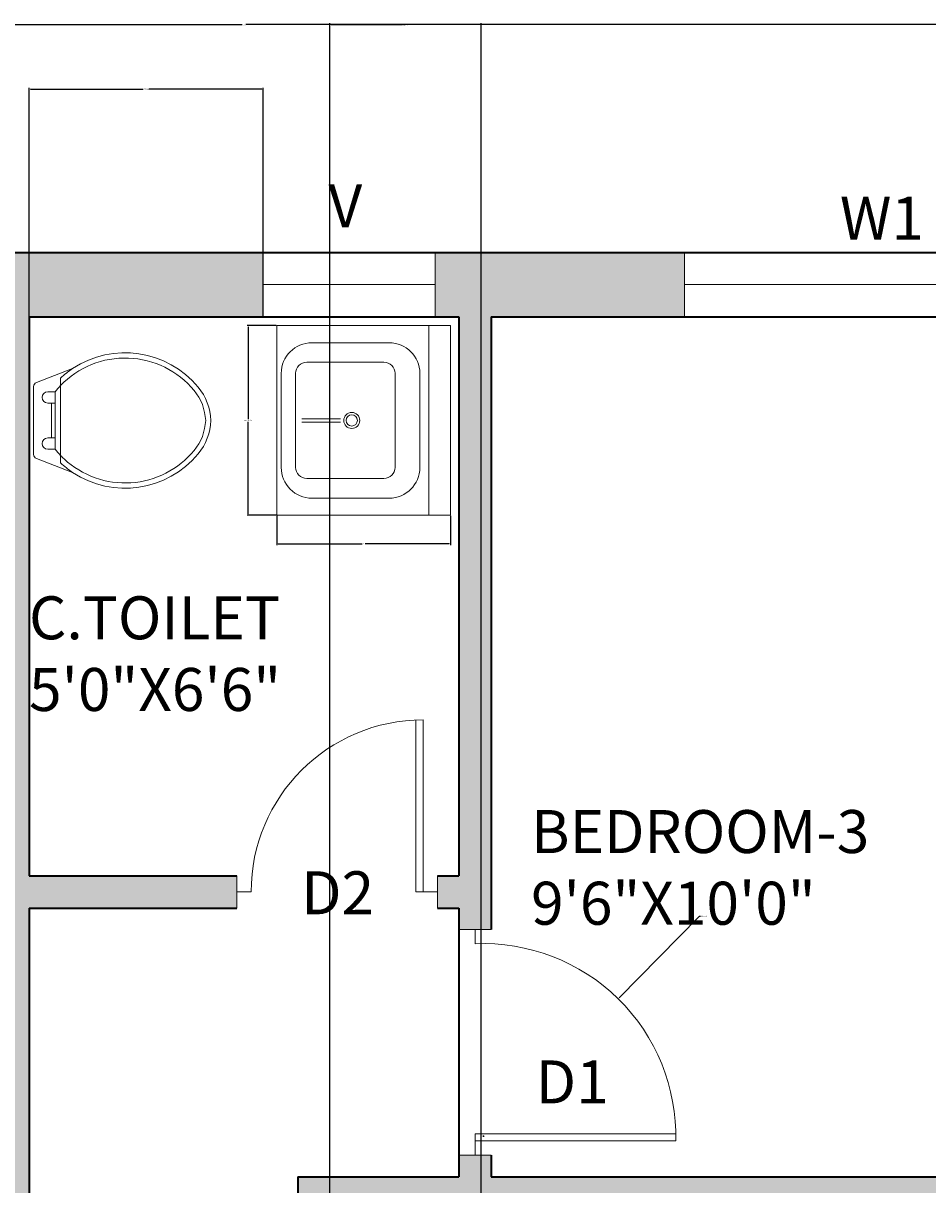
# Model space of a CAD drawing. Units: inches. Extents: x 5 to 421, y -617 to 43.
# Tile 14 of 15: x 182 to 308, y -119 to 43. Entities that reach past the tile are written whole.
import ezdxf

# ---------------------------------------------------------------- set-up
doc = ezdxf.new("R2010")
doc.units = ezdxf.units.IN
doc.header["$MEASUREMENT"] = 0
for name, color, linetype, lineweight in [('A-ANNO-DIMS', 2, 'Continuous', 18), ('A-ANNO-TEXT', 7, 'Continuous', 18), ('A-AREA-IDEN', 7, 'Continuous', 25), ('A-DOOR', 4, 'Continuous', 20), ('A-FLOR-FIXT', 9, 'Continuous', 18), ('A-GLAZ', 4, 'Continuous', 18), ('A-WALL', 7, 'Continuous', 35), ('WC-Detail_dwgmodels.com', 251, 'Continuous', 13), ('WC-Outline_dwgmodels.com', 250, 'Continuous', 18)]:
    doc.layers.add(name, color=color, linetype=linetype, lineweight=lineweight)
doc.layers.add('A-WALL-PATT', color=251, linetype='Continuous', lineweight=13, true_color=0x636466)
doc.styles.get("Standard").update_dxf_attribs({"font": 'arial.ttf'})
doc.dimstyles.get("Standard").update_dxf_attribs({"dimtxt": 0.18, "dimasz": 0.18, "dimexe": 0.18, "dimexo": 0.0625, "dimgap": 0.09, "dimtad": 0, "dimtih": 1, "dimtoh": 1, "dimdec": 0, "dimzin": 0, "dimdsep": 46, "dimlunit": 3, "dimtxsty": 'Standard', "dimcen": 0.09, "dimadec": 0, "dimazin": 0, "dimtfac": 1, "dimtdec": 0, "dimtofl": 0, "dimtmove": 0, "dimatfit": 3, "dimfxl": 1, "dimtolj": 1, "dimtzin": 0, "dimarcsym": 0})

# ---------------------------------------------------------------- blocks, each defined once
blk = doc.blocks.new('М14 600х655')
for p, q in [((-655, 600), (-655, 0)), ((-655, 600), (-655, 0)), ((-655, 0), (-655, 600)), ((0, 600), (-655, 600)), ((0, 0), (0, 600)), ((0, 525), (-655, 525)), ((-165.1, 494.1), (-489.9, 494.1)), ((-165.4, 408.4), (-490.2, 408.4)), ((-595.8, 388.1), (-595.8, 121.3)), ((-528.4, 370.1), (-528.4, 103.3)), ((-127.2, 103.3), (-127.2, 370.1)), ((-59.2, 121.3), (-59.2, 388.1)), ((-333.5, 87.1), (-333.5, 219.6)), ((-321.5, 87.1), (-321.5, 219.6)), ((-490.2, 65.1), (-165.4, 65.1)), ((-655, 0), (-655, 0)), ((-655, 0), (-655, 0)), ((-655, 0), (0, 0)), ((-655, 0), (0, 0)), ((-489.9, 15.4), (-165.1, 15.4))]:
    blk.add_line(p, q)
for radius in [27.6, 19.3]:
    blk.add_circle((-327.5, 258.9), radius)
for centre, radius, start, end in [((-489.9, 388.1), 105.9, 90, 180), ((-165.1, 388.1), 105.9, 0, 90), ((-490.2, 370.1), 38.2, 90, 180), ((-165.4, 370.1), 38.2, 0, 90), ((-489.9, 121.3), 105.9, 180, 270), ((-165.1, 121.3), 105.9, 270, 0), ((-490.2, 103.3), 38.2, 180, 270), ((-165.4, 103.3), 38.2, 270, 0)]:
    blk.add_arc(centre, radius, start, end)
blk = doc.blocks.new('VENT-24')
for p, q in [((0, 9), (24, 9)), ((0, 0), (0, 9)), ((24, 9), (24, 0)), ((0, 4.5), (24, 4.5)), ((24, 0), (0, 0))]:
    blk.add_line(p, q)
blk = doc.blocks.new('WINDOW-W1-60')
for p, q in [((0, 9), (60, 9)), ((0, 0), (0, 9)), ((60, 9), (60, 0)), ((0, 4.5), (60, 4.5)), ((60, 0), (0, 0))]:
    blk.add_line(p, q)
blk = doc.blocks.new('DOOR-SWING-24')
for p, q in [((23, 0), (23, 24)), ((24, 0), (24, 24))]:
    blk.add_line(p, q)
blk.add_arc((24, 0), 24, 90, 180)
blk = doc.blocks.new('*D38')
at = {"layer": 'A-ANNO-DIMS', "color": 0, "lineweight": -2, "transparency": 16777216}
for p, q in [((217.43, 0.66), (213.34, 0.66)), ((213.52, 0.48), (213.52, -12.39)), ((213.52, -25.63), (213.52, -12.76)), ((217.43, -25.81), (213.34, -25.81))]:
    blk.add_line(p, q, dxfattribs=at)
at = {"layer": 'A-ANNO-DIMS', "color": 0, "transparency": 16777216}
for points in [[(213.49, 0.48), (213.55, 0.48), (213.52, 0.66)], [(213.49, -25.63), (213.55, -25.63), (213.52, -25.81)]]:
    blk.add_solid(points, dxfattribs=at)
at = {"layer": 'Defpoints', "color": 0, "transparency": 16777216}
for p in [(217.49, 0.66), (213.52, -25.81), (217.49, -25.81)]:
    blk.add_point(p, dxfattribs=at)
at = {"layer": 'A-ANNO-DIMS', "color": 0, "transparency": 16777216, "insert": (213.52, -12.58), "char_height": 0.18, "attachment_point": 5}
blk.add_mtext('\\A1;BASIN 26', dxfattribs=at)
blk = doc.blocks.new('*D39')
at = {"layer": 'A-ANNO-DIMS', "color": 0, "lineweight": -2, "transparency": 16777216}
for p, q in [((217.49, -25.88), (217.49, -29.97)), ((241.75, -25.88), (241.75, -29.97)), ((217.67, -29.79), (229.4, -29.79)), ((241.57, -29.79), (229.84, -29.79))]:
    blk.add_line(p, q, dxfattribs=at)
at = {"layer": 'A-ANNO-DIMS', "color": 0, "transparency": 16777216}
for points in [[(217.67, -29.76), (217.67, -29.82), (217.49, -29.79)], [(241.57, -29.76), (241.57, -29.82), (241.75, -29.79)]]:
    blk.add_solid(points, dxfattribs=at)
at = {"layer": 'Defpoints', "color": 0, "transparency": 16777216}
for p in [(217.49, -25.81), (241.75, -25.81), (241.75, -29.79)]:
    blk.add_point(p, dxfattribs=at)
at = {"layer": 'A-ANNO-DIMS', "color": 0, "transparency": 16777216, "insert": (229.62, -29.79), "char_height": 0.18, "attachment_point": 5}
blk.add_mtext('\\A1;24', dxfattribs=at)
blk = doc.blocks.new('*D54')
at = {"layer": 'A-ANNO-DIMS', "color": 0, "lineweight": -2, "transparency": 16777216}
for p, q in [((37.42, 10.94), (37.42, 42.86)), ((37.6, 42.68), (212.65, 42.68)), ((388.24, 42.68), (213.19, 42.68)), ((388.42, -118.06), (388.42, 42.86))]:
    blk.add_line(p, q, dxfattribs=at)
at = {"layer": 'A-ANNO-DIMS', "color": 0, "transparency": 16777216}
for points in [[(37.6, 42.71), (37.6, 42.65), (37.42, 42.68)], [(388.24, 42.71), (388.24, 42.65), (388.42, 42.68)]]:
    blk.add_solid(points, dxfattribs=at)
at = {"layer": 'Defpoints', "color": 0, "transparency": 16777216}
for p in [(37.42, 42.68), (37.42, 10.88), (388.42, -118.12)]:
    blk.add_point(p, dxfattribs=at)
at = {"layer": 'A-ANNO-DIMS', "color": 0, "transparency": 16777216, "insert": (212.92, 42.68), "char_height": 0.18, "attachment_point": 5}
blk.add_mtext('\\A1;351', dxfattribs=at)
blk = doc.blocks.new('*D55')
at = {"layer": 'A-ANNO-DIMS', "color": 0, "lineweight": -2, "transparency": 16777216}
for p, q in [((370.48, 10.88), (420.4, 10.88)), ((420.22, 10.7), (420.22, -286.69)), ((420.22, -584.44), (420.22, -287.05)), ((169.48, -584.62), (420.4, -584.62))]:
    blk.add_line(p, q, dxfattribs=at)
at = {"layer": 'A-ANNO-DIMS', "color": 0, "transparency": 16777216}
for points in [[(420.19, 10.7), (420.25, 10.7), (420.22, 10.88)], [(420.19, -584.44), (420.25, -584.44), (420.22, -584.62)]]:
    blk.add_solid(points, dxfattribs=at)
at = {"layer": 'Defpoints', "color": 0, "transparency": 16777216}
for p in [(370.42, 10.88), (169.42, -584.62), (420.22, -584.62)]:
    blk.add_point(p, dxfattribs=at)
at = {"layer": 'A-ANNO-DIMS', "color": 0, "transparency": 16777216, "insert": (420.22, -286.87), "char_height": 0.18, "attachment_point": 5}
blk.add_mtext('\\A1;595.5', dxfattribs=at)
blk = doc.blocks.new('*D57')
at = {"layer": 'A-ANNO-DIMS', "color": 0, "lineweight": -2, "transparency": 16777216}
for p, q in [((182.92, 1.94), (182.92, 33.86)), ((183.1, 33.68), (198.86, 33.68)), ((215.42, 33.68), (199.65, 33.68)), ((215.6, 1.94), (215.6, 33.86))]:
    blk.add_line(p, q, dxfattribs=at)
at = {"layer": 'A-ANNO-DIMS', "color": 0, "transparency": 16777216}
for points in [[(183.1, 33.71), (183.1, 33.65), (182.92, 33.68)], [(215.42, 33.71), (215.42, 33.65), (215.6, 33.68)]]:
    blk.add_solid(points, dxfattribs=at)
at = {"layer": 'Defpoints', "color": 0, "transparency": 16777216}
for p in [(215.6, 33.68), (182.92, 1.88), (215.6, 1.88)]:
    blk.add_point(p, dxfattribs=at)
at = {"layer": 'A-ANNO-DIMS', "color": 0, "transparency": 16777216, "insert": (199.26, 33.68), "char_height": 0.18, "attachment_point": 5}
blk.add_mtext('\\A1;32.68', dxfattribs=at)
blk = doc.blocks.new('*D71')
at = {"layer": 'A-ANNO-DIMS', "color": 0, "lineweight": -2, "transparency": 16777216}
for p, q in [((224.92, -122.56), (224.92, 42.86)), ((225.1, 42.68), (235.06, 42.68)), ((245.82, 42.68), (235.85, 42.68)), ((246, -128.12), (246, 42.86))]:
    blk.add_line(p, q, dxfattribs=at)
at = {"layer": 'A-ANNO-DIMS', "color": 0, "transparency": 16777216}
for points in [[(225.1, 42.71), (225.1, 42.65), (224.92, 42.68)], [(245.82, 42.71), (245.82, 42.65), (246, 42.68)]]:
    blk.add_solid(points, dxfattribs=at)
at = {"layer": 'Defpoints', "color": 0, "transparency": 16777216}
for p in [(246, 42.68), (224.92, -122.62), (246, -128.18)]:
    blk.add_point(p, dxfattribs=at)
at = {"layer": 'A-ANNO-DIMS', "color": 0, "transparency": 16777216, "insert": (235.46, 42.68), "char_height": 0.18, "attachment_point": 5}
blk.add_mtext('\\A1;21.08', dxfattribs=at)
blk = doc.blocks.new('*D79')
at = {"layer": 'A-ANNO-DIMS', "color": 0, "lineweight": -2, "transparency": 16777216}
for p, q in [((276.43, -81.8), (265.27, -93.16)), ((276.61, -81.8), (276.43, -81.8)), ((246.25, -112.44), (246.43, -112.44)), ((246.34, -112.53), (246.34, -112.35))]:
    blk.add_line(p, q, dxfattribs=at)
at = {"layer": 'A-ANNO-DIMS', "color": 0, "transparency": 16777216}
blk.add_solid([(265.25, -93.14), (265.29, -93.18), (265.14, -93.29)], dxfattribs=at)
at = {"layer": 'Defpoints', "color": 0, "transparency": 16777216}
for p in [(265.14, -93.29), (246.34, -112.44)]:
    blk.add_point(p, dxfattribs=at)
at = {"layer": 'A-ANNO-DIMS', "color": 0, "transparency": 16777216, "insert": (277.09, -81.8), "char_height": 0.18, "attachment_point": 5}
blk.add_mtext('\\A1;R26.84', dxfattribs=at)

msp = doc.modelspace()

# ---------------------------------------------------------------- hatches: boundary and pattern name
at = {"layer": 'A-WALL-PATT'}
h = msp.add_hatch(color=256, dxfattribs=at)
h.dxf.hatch_style = 1
h.paths.add_polyline_path([(46.4196, -88.1188), (37.4196, -88.1188), (37.4196, -166.6119), (46.4196, -166.6119), (46.4196, -122.6188), (135.4196, -122.6188), (135.4196, -120.3688), (135.4196, -118.1188), (46.4196, -118.1188)])
h.paths.add_polyline_path([(82.4196, 10.8812), (37.4196, 10.8812), (37.4196, -28.1188), (46.4196, -28.1188), (46.4196, 1.8812), (82.4196, 1.8812)])
h.paths.add_polyline_path([(215.5968, 10.8812), (142.4196, 10.8812), (142.4196, 1.8812), (178.4196, 1.8812), (178.4196, -118.1188), (175.4196, -118.1188), (175.4196, -122.6188), (182.9196, -122.6188), (182.9196, -80.6188), (211.9196, -80.6188), (211.9196, -78.3688), (211.9196, -76.1188), (182.9196, -76.1188), (182.9196, 1.8812), (215.5968, 1.8812)])
h.paths.add_polyline_path([(274.4196, 10.8812), (239.5968, 10.8812), (239.5968, 1.8812), (242.9196, 1.8812), (242.9196, -76.1188), (239.9196, -76.1188), (239.9196, -80.6188), (242.9196, -80.6188), (242.9196, -83.6188), (247.4196, -83.6188), (247.4196, 1.8812), (274.4196, 1.8812)])
h.paths.add_polyline_path([(370.4196, 10.8812), (334.4196, 10.8812), (334.4196, 1.8812), (361.4196, 1.8812), (361.4196, -28.1188), (370.4196, -28.1188)])
h.paths.add_polyline_path([(370.4196, -88.1188), (361.4196, -88.1188), (361.4196, -118.1188), (247.4196, -118.1188), (247.4196, -115.1188), (242.9196, -115.1188), (242.9196, -118.1188), (220.4196, -118.1188), (220.4196, -158.6188), (224.9196, -158.6188), (224.9196, -122.6188), (326.9196, -122.6188), (326.9196, -170.7662), (331.4196, -170.7662), (331.4196, -122.6188), (370.4196, -122.6188)])
h.paths.add_polyline_path([(388.4196, -122.6188), (388.4196, -118.1188), (379.4196, -118.1188), (379.4196, -122.6188), (379.4196, -154.8688), (388.4196, -154.8688)])
h.paths.add_polyline_path([(388.4196, -214.8688), (379.4196, -214.8688), (379.4196, -247.1188), (388.4196, -247.1188)])
h.paths.add_polyline_path([(371.0265, -242.6188), (331.4196, -242.6188), (331.4196, -239.6188), (326.9196, -239.6188), (326.9196, -242.6188), (224.9196, -242.6188), (224.9196, -206.6188), (220.4196, -206.6188), (220.4196, -343.6188), (224.9196, -343.6188), (229.4196, -343.6188), (229.4196, -247.1188), (261.5265, -247.1188), (261.5265, -276.1188), (263.7765, -276.1188), (266.0265, -276.1188), (266.0265, -247.1188), (362.0265, -247.1188), (362.0265, -265.1188), (371.0265, -265.1188), (371.0265, -247.1188)])
h.paths.add_polyline_path([(371.0265, -289.1188), (362.0265, -289.1188), (362.0265, -307.1188), (266.0265, -307.1188), (266.0265, -304.1188), (261.5265, -304.1188), (261.5265, -307.1188), (261.5265, -311.6188), (362.0265, -311.6188), (362.0265, -353.6188), (371.0265, -353.6188)])
h.paths.add_polyline_path([(371.0265, -413.6188), (362.0265, -413.6188), (362.0265, -455.6188), (325.7231, -455.6188), (325.7231, -464.6188), (361.4196, -464.6188), (371.0265, -464.6188)])
h.paths.add_polyline_path([(265.7231, -455.6188), (229.4196, -455.6188), (229.4196, -383.6188), (220.4196, -383.6188), (220.4196, -386.6188), (207.4649, -386.6188), (207.4649, -395.6188), (220.4196, -395.6188), (220.4196, -455.6188), (216.0568, -455.6188), (216.0568, -464.6188), (265.7231, -464.6188)])
h.paths.add_polyline_path([(169.4196, -386.6188), (137.9196, -386.6188), (137.9196, -395.6188), (160.4196, -395.6188), (160.4196, -424.2032), (169.4196, -424.2032)])
h.paths.add_polyline_path([(169.4196, -453.7423), (160.4196, -453.7423), (160.4196, -464.6188), (169.4196, -464.6188)])
h.paths.add_polyline_path([(46.4196, -575.6188), (37.4196, -575.6188), (37.4196, -584.6188), (46.4196, -584.6188)])
h.paths.add_polyline_path([(169.4196, -575.6188), (160.4196, -575.6188), (160.4196, -579.5504), (160.4196, -584.6188), (169.4196, -584.6188)])
h.paths.add_polyline_path([(46.4196, -226.6119), (37.4196, -226.6119), (37.4196, -292.8008), (46.4196, -292.8008)])
h.paths.add_polyline_path([(46.4196, -352.8008), (37.4196, -352.8008), (37.4196, -395.6188), (77.9196, -395.6188), (77.9196, -386.6188), (46.4196, -386.6188)])

# ---------------------------------------------------------------- linework, layer by layer
at = {"layer": 'A-DOOR'}
for p, q in [((211.9196, -78.3688), (211.9196, -76.1188)), ((239.9196, -76.1188), (239.9196, -80.6188)), ((213.9196, -78.3688), (211.9196, -78.3688)), ((211.9196, -78.3688), (211.9196, -80.6188)), ((239.9196, -78.3688), (236.9196, -78.3688)), ((242.9196, -83.6188), (247.4196, -83.6188)), ((245.1696, -83.6188), (245.1696, -85.6188)), ((245.1696, -115.1188), (245.1696, -112.1188)), ((245.1696, -112.1188), (273.1696, -112.1188)), ((245.1696, -113.1188), (273.1696, -113.1188)), ((242.9196, -115.1188), (247.4196, -115.1188))]:
    msp.add_line(p, q, dxfattribs=at)
msp.add_arc((246.3366, -112.4351), 26.8417, 358.540409, 92.49192, dxfattribs=at)
at = {"layer": 'A-WALL'}
for p, q in [((37.4196, 10.8812), (370.4196, 10.8812)), ((182.9196, 1.8812), (182.9196, -76.1188)), ((182.9196, 1.8812), (242.9196, 1.8812)), ((242.9196, 1.8812), (242.9196, -76.1188)), ((247.4196, 1.8812), (247.4196, -83.6188)), ((247.4196, 1.8812), (361.4196, 1.8812)), ((182.9196, -76.1188), (211.9196, -76.1188)), ((239.9196, -76.1188), (242.9196, -76.1188)), ((182.9196, -80.6188), (211.9196, -80.6188)), ((182.9196, -80.6188), (182.9196, -122.6188)), ((239.9196, -80.6188), (242.9196, -80.6188)), ((242.9196, -80.6188), (242.9196, -118.1188)), ((247.4196, -115.1188), (247.4196, -118.1188)), ((220.4196, -118.1188), (242.9196, -118.1188)), ((220.4196, -118.1188), (220.4196, -158.6188)), ((247.4196, -118.1188), (361.4196, -118.1188))]:
    msp.add_line(p, q, dxfattribs=at)
at = {"layer": 'WC-Detail_dwgmodels.com'}
for p, q in [((187.3057, -7.7101), (187.3057, -6.6717)), ((187.3057, -18.489), (187.3057, -17.4506))]:
    msp.add_line(p, q, dxfattribs=at)
for points in [[(187.3057, -6.6717, -0.04093657), (189.0045, -5.3315, -0.16373228)], [(186.5584, -8.564, -0.02271164), (187.3057, -7.7101, -0.16261828)], [(186.5584, -8.564), (185.5193, -8.564, 1), (185.5193, -10.143), (186.0601, -10.143)], [(186.5584, -12.5804), (186.5584, -8.564, -0.47610764)], [(186.5584, -12.5804), (186.5584, -16.5967, 0.02271164)], [(186.5584, -16.5967), (185.5193, -16.5967, -1), (185.5193, -15.0177), (186.0601, -15.0177)], [(186.5584, -16.5967, 0.02271164), (187.3057, -17.4506, 0.16261828)], [(187.3057, -18.489, 0.04093657), (189.0045, -19.8292, 0.16373228)]]:
    msp.add_lwpolyline(points, format="xyb", dxfattribs=at)
for points in [[(186.0601, -10.143), (186.0601, -15.0177)], [(186.0601, -10.143), (186.5584, -10.143)], [(186.0601, -15.0177), (186.5584, -15.0177)]]:
    msp.add_lwpolyline(points, dxfattribs=at)
at = {"layer": 'WC-Outline_dwgmodels.com'}
for p in [(187.3057, -7.7101), (187.3057, -17.4506)]:
    msp.add_line(p, (187.3057, -12.5804), dxfattribs=at)
for points in [[(189.0045, -5.3315, -0.38391851), (206.5293, -7.9269, -0.16373228), (208.3131, -12.5804, -0.35973259)], [(187.3057, -7.7101, -0.44854579), (205.9589, -8.3982, -0.16261828), (207.5725, -12.5804, -0.47087745)], [(183.5577, -12.5804), (183.5577, -7.8532, -0.31031032), (183.9556, -7.2738), (189.0045, -5.3315, -0.20907131)], [(183.5577, -12.5804), (183.5577, -17.3075, 0.31031032), (183.9556, -17.8869), (189.0045, -19.8292, 0.20907131)], [(187.8099, -17.9475, 0.43163885), (205.9589, -16.7625, 0.16261828), (207.5725, -12.5804, 0.47087745)], [(189.0045, -19.8292, 0.38391851), (206.5293, -17.2339, 0.16373228), (208.3131, -12.5804, 0.35973259)], [(187.3057, -17.4506, 0.01416454), (187.8099, -17.9475, 0.16261828)]]:
    msp.add_lwpolyline(points, format="xyb", dxfattribs=at)

# ---------------------------------------------------------------- block references
at = {"layer": 'A-DOOR'}
msp.add_blockref('DOOR-SWING-24', (213.9196, -78.3688), dxfattribs=at)
at = {"layer": 'A-FLOR-FIXT', "xscale": 0.0404235432921695, "yscale": 0.0404235432921695, "zscale": 0.0404235432921695, "rotation": 270}
msp.add_blockref('М14 600х655', (217.4921, -25.8141), dxfattribs=at)
at = {"layer": 'A-GLAZ'}
for name, p in [('VENT-24', (215.5968, 1.8812)), ('WINDOW-W1-60', (274.4196, 1.8812))]:
    msp.add_blockref(name, p, dxfattribs=at)

# ---------------------------------------------------------------- texts
at = {"layer": 'A-ANNO-TEXT', "char_height": 6, "attachment_point": 1}
for s, width, insert in [('V', 0.328709, (224.705, 20.36)), ('W1', 0.387986, (296.0884, 18.6451)), ('D1', 2.046076, (253.6398, -101.8857))]:
    msp.add_mtext_dynamic_manual_height_columns(s, width=width, gutter_width=1, heights=[0], dxfattribs=dict(at, insert=insert))
at = {"layer": 'A-ANNO-TEXT', "insert": (220.9024, -75.4945), "char_height": 6, "attachment_point": 1}
msp.add_mtext('D2', dxfattribs=at)
at = {"layer": 'A-AREA-IDEN', "insert": (182.9196, -37.1188), "char_height": 6, "attachment_point": 1}
msp.add_mtext_dynamic_manual_height_columns('C.TOILET\\P5\'0"X6\'6"', width=0.372014, gutter_width=1, heights=[0], dxfattribs=at)
at = {"layer": 'A-AREA-IDEN', "insert": (252.9859, -66.9501), "char_height": 6, "attachment_point": 1}
msp.add_mtext('BEDROOM-3\\P9\'6"X10\'0"', dxfattribs=at)

# ---------------------------------------------------------------- dimensions: what is measured, and where the dimension line sits
at = {"layer": 'A-ANNO-DIMS'}
for base, p1, p2, override, picture, middle in [((37.4196, 42.6812), (388.4196, -118.1188), (37.4196, 10.8812), {"dimdec": 0, "dimlfac": 1, "dimrnd": 0, "dimzin": 0, "dimdsep": 46, "dimlunit": 2}, '*D54', (212.9196, 42.6812)), ((245.9983, 42.6812), (224.9196, -122.6188), (245.9983, -128.1837), {"dimdec": 2, "dimlfac": 1, "dimrnd": 0, "dimzin": 0, "dimdsep": 46, "dimlunit": 2}, '*D71', (235.4589, 42.6812)), ((241.7462, -29.7857), (217.4921, -25.8141), (241.7462, -25.8141), {"dimdec": 0, "dimlfac": 1, "dimrnd": 0, "dimzin": 0, "dimdsep": 46, "dimlunit": 2}, '*D39', (229.6192, -29.7857))]:
    dim = msp.add_linear_dim(base=base, p1=p1, p2=p2, dimstyle='Standard', override=override, dxfattribs=at)
    dim.commit()
    dim.dimension.update_dxf_attribs({"geometry": picture, "text_midpoint": middle})
for base, p1, p2, angle, override, picture, middle in [((215.5968, 33.6812), (182.9196, 1.8812), (215.5968, 1.8812), 0, {"dimdec": 2, "dimlfac": 1, "dimrnd": 0, "dimzin": 0, "dimdsep": 46, "dimlunit": 2}, '*D57', (199.2582, 33.6812)), ((420.2196, -584.6188), (370.4196, 10.8812), (169.4196, -584.6188), 90, {"dimdec": 1, "dimlfac": 1, "dimrnd": 0, "dimzin": 0, "dimdsep": 46, "dimlunit": 2}, '*D55', (420.2196, -286.8688))]:
    dim = msp.add_linear_dim(base=base, p1=p1, p2=p2, angle=angle, dimstyle='Standard', override=override, dxfattribs=at)
    dim.commit()
    dim.dimension.update_dxf_attribs({"geometry": picture, "text_midpoint": middle})
dim = msp.add_linear_dim(base=(213.5205, -25.8141), p1=(217.4921, 0.6633), p2=(217.4921, -25.8141), angle=270, text='BASIN <>', dimstyle='Standard', override={"dimdec": 0, "dimlfac": 1, "dimrnd": 0, "dimzin": 0, "dimdsep": 46, "dimlunit": 2}, dxfattribs=at)
dim.commit()
dim.dimension.update_dxf_attribs({"geometry": '*D38', "text_midpoint": (213.5205, -12.5754)})
dim = msp.add_radius_dim(center=(246.3366, -112.4351), mpoint=(265.1449, -93.2851), dimstyle='Standard', override={"dimdec": 2, "dimlfac": 1, "dimrnd": 0, "dimzin": 0, "dimdsep": 46, "dimlunit": 2}, dxfattribs=at)
dim.commit()
dim.dimension.update_dxf_attribs({"geometry": '*D79', "text_midpoint": (277.0894, -81.7951), "dimtype": 164})

doc.saveas('drawing.dxf')
